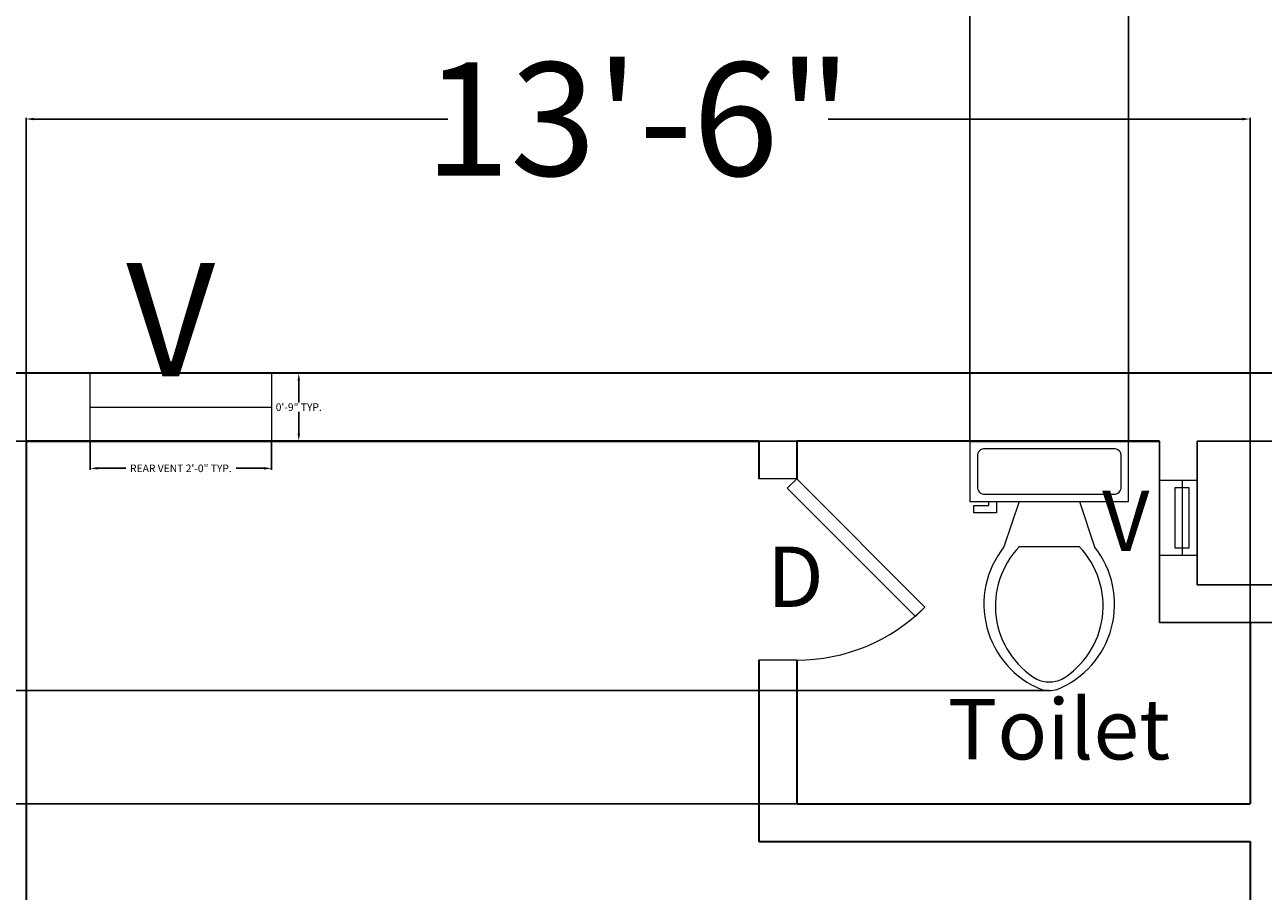
# Model space of a CAD drawing. Units: inches. Extents: x 371 to 1095, y -45 to 1219.
# Tile 16 of 18: x 502 to 666, y 913 to 1028. Entities that reach past the tile are written whole.
import ezdxf

# ---------------------------------------------------------------- set-up
doc = ezdxf.new("R2010")
doc.units = ezdxf.units.IN
doc.header["$MEASUREMENT"] = 0
for name, color, linetype, lineweight in [('A-ANNO-DIMS', 2, 'Continuous', 18), ('A-ANNO-TEXT', 7, 'Continuous', 18), ('A-AREA-IDEN', 7, 'Continuous', 18), ('A-DOOR', 3, 'Continuous', 18), ('A-FLOR-FIXT', 9, 'Continuous', 18), ('A-FLOR-SHFT', 7, 'Continuous', 25), ('A-GLAZ', 4, 'Continuous', 18), ('A-WALL', 40, 'Continuous', 35)]:
    doc.layers.add(name, color=color, linetype=linetype, lineweight=lineweight)
doc.styles.get("Standard").update_dxf_attribs({"font": 'arial.ttf'})
doc.dimstyles.get("Standard").update_dxf_attribs({"dimtxt": 1, "dimasz": 1, "dimexe": 0.18, "dimexo": 0.0625, "dimgap": 0.09, "dimtad": 0, "dimtih": 1, "dimtoh": 1, "dimdec": 0, "dimzin": 0, "dimdsep": 46, "dimlunit": 3, "dimtxsty": 'Standard', "dimcen": 0.09, "dimadec": 0, "dimazin": 0, "dimtfac": 1, "dimtdec": 0, "dimtofl": 0, "dimtmove": 0, "dimatfit": 3, "dimfxl": 1, "dimtolj": 1, "dimtzin": 0, "dimarcsym": 0})

# ---------------------------------------------------------------- blocks, each defined once
blk = doc.blocks.new('*U2')
for p, q in [((9.5, -6), (9.5, -2)), ((-8, -8.5), (-8, -8)), ((-7, -8), (-7, -9.5)), ((-4, -8), (-6, -14)), ((4, -8), (6, -14)), ((-10, -8.5), (-8, -8.5)), ((-10, -9.5), (-10, -8.5)), ((-7, -9.5), (-10, -9.5)), ((4, -14), (-4, -14))]:
    blk.add_line(p, q)
blk.add_lwpolyline([(10.5, -8), (10.5, 0), (-10.5, 0), (-10.5, -8)], close=True)
for points in [[(8.5, -1), (-8.5, -1)], [(-9.5, -2), (-9.5, -6)], [(-8.5, -7), (8.5, -7)]]:
    blk.add_lwpolyline(points)
for centre, radius, start, end in [((-8.62, -1.88), 0.884, 81.8699, 188.1301), ((8.62, -1.88), 0.884, 351.8699, 98.1301), ((-8.62, -6.12), 0.884, 171.8699, 278.1301), ((8.62, -6.12), 0.884, 261.8699, 8.1301), ((3.52, -21.58), 12.17, 141.4691, 247.9714), ((4.2, -21.82), 11.33, 136.3677, 238.9468), ((-3.52, -21.58), 12.17, 292.0284, 38.5307), ((-4.2, -21.82), 11.33, 301.053, 43.6321), ((0, -27.88), 4, 245.7318, 294.2682), ((0, -29), 4, 254.8605, 285.1395)]:
    blk.add_arc(centre, radius, start, end)
blk = doc.blocks.new('*U5')
for p, q in [((0, 0), (0, -5)), ((24, 0), (24, -5))]:
    blk.add_line(p, q)
blk.add_lwpolyline([(0, 0), (16.97, 16.97), (18.21, 15.73), (1.24, -1.24)], close=True)
blk.add_arc((0, 0), 24, 0, 45)
blk = doc.blocks.new('*D8')
at = {"layer": 'A-ANNO-DIMS', "color": 0, "lineweight": -2, "transparency": 16777216}
for p, q in [((501.75, 973.03), (438.47, 973.03)), ((438.65, 972.03), (438.65, 896.65)), ((438.65, 806.03), (438.65, 881.4)), ((501.75, 805.03), (438.47, 805.03))]:
    blk.add_line(p, q, dxfattribs=at)
at = {"layer": 'A-ANNO-DIMS', "color": 0, "transparency": 16777216}
for points in [[(438.48, 972.03), (438.82, 972.03), (438.65, 973.03)], [(438.48, 806.03), (438.82, 806.03), (438.65, 805.03)]]:
    blk.add_solid(points, dxfattribs=at)
at = {"layer": 'Defpoints', "color": 0, "transparency": 16777216}
for p in [(501.81, 973.03), (438.65, 805.03), (501.81, 805.03)]:
    blk.add_point(p, dxfattribs=at)
at = {"layer": 'A-ANNO-DIMS', "color": 0, "transparency": 16777216, "insert": (438.65, 889.03), "char_height": 1, "attachment_point": 5}
blk.add_mtext("\\A1;{\\H15x;14'}", dxfattribs=at)
blk = doc.blocks.new('*D19')
at = {"layer": 'A-ANNO-DIMS', "color": 0, "lineweight": -2, "transparency": 16777216}
for p, q in [((501.75, 982.03), (438.6, 982.03)), ((438.78, 981.03), (438.78, 974.03)), ((438.78, 972.03), (437.78, 972.03)), ((501.75, 973.03), (438.6, 973.03)), ((438.78, 973.03), (438.78, 972.03))]:
    blk.add_line(p, q, dxfattribs=at)
at = {"layer": 'A-ANNO-DIMS', "color": 0, "transparency": 16777216}
for points in [[(438.62, 981.03), (438.95, 981.03), (438.78, 982.03)], [(438.62, 974.03), (438.95, 974.03), (438.78, 973.03)]]:
    blk.add_solid(points, dxfattribs=at)
at = {"layer": 'Defpoints', "color": 0, "transparency": 16777216}
for p in [(501.81, 982.03), (438.78, 973.03), (501.81, 973.03)]:
    blk.add_point(p, dxfattribs=at)
at = {"layer": 'A-ANNO-DIMS', "color": 0, "transparency": 16777216, "insert": (429.07, 972.03), "char_height": 1, "attachment_point": 5}
blk.add_mtext('\\A1;{\\H15x;9"}', dxfattribs=at)
blk = doc.blocks.new('*D26')
at = {"layer": 'A-ANNO-DIMS', "color": 0, "lineweight": -2, "transparency": 16777216}
for p, q in [((501.81, 949.09), (501.81, 1015.85)), ((502.81, 1015.67), (557.66, 1015.67)), ((662.81, 1015.67), (607.96, 1015.67)), ((663.81, 949.09), (663.81, 1015.85))]:
    blk.add_line(p, q, dxfattribs=at)
at = {"layer": 'A-ANNO-DIMS', "color": 0, "transparency": 16777216}
for points in [[(502.81, 1015.84), (502.81, 1015.51), (501.81, 1015.67)], [(662.81, 1015.84), (662.81, 1015.51), (663.81, 1015.67)]]:
    blk.add_solid(points, dxfattribs=at)
at = {"layer": 'Defpoints', "color": 0, "transparency": 16777216}
for p in [(501.81, 1015.67), (501.81, 949.03), (663.81, 949.03)]:
    blk.add_point(p, dxfattribs=at)
at = {"layer": 'A-ANNO-DIMS', "color": 0, "transparency": 16777216, "insert": (582.81, 1015.67), "char_height": 1, "attachment_point": 5}
blk.add_mtext('\\A1;{\\H15x;13\'-6"}', dxfattribs=at)
blk = doc.blocks.new('VENT-24-REAR')
blk.add_line((0, 4.5), (24, 4.5))
blk.add_lwpolyline([(0, 9), (24, 9), (24, 0), (0, 0)], close=True)
blk = doc.blocks.new('VENT-DUCT-SASH')
blk.add_line((0.9, 10), (0.9, 0))
blk.add_lwpolyline([(1.79, 9), (1.79, 1), (0, 1), (0, 9)], close=True)
blk = doc.blocks.new('SHAFT-REAR')
for p, q in [((0, 24), (0, 0)), ((5, 24), (5, 5)), ((28, 24), (5, 24)), ((28, 24), (28, 5)), ((33, 24), (33, 0)), ((5, 5), (28, 5)), ((0, 0), (33, 0))]:
    blk.add_line(p, q)
blk = doc.blocks.new('*D40')
at = {"layer": 'A-ANNO-DIMS', "color": 0, "lineweight": -2, "transparency": 16777216}
for p, q in [((510.31, 972.96), (510.31, 969.25)), ((534.31, 972.96), (534.31, 969.25)), ((511.31, 969.43), (515.01, 969.43)), ((533.31, 969.43), (529.62, 969.43))]:
    blk.add_line(p, q, dxfattribs=at)
at = {"layer": 'A-ANNO-DIMS', "color": 0, "transparency": 16777216}
for points in [[(511.31, 969.59), (511.31, 969.26), (510.31, 969.43)], [(533.31, 969.59), (533.31, 969.26), (534.31, 969.43)]]:
    blk.add_solid(points, dxfattribs=at)
at = {"layer": 'Defpoints', "color": 0, "transparency": 16777216}
for p in [(510.31, 973.03), (534.31, 973.03), (534.31, 969.43)]:
    blk.add_point(p, dxfattribs=at)
at = {"layer": 'A-ANNO-DIMS', "color": 0, "transparency": 16777216, "insert": (522.31, 969.43), "char_height": 1, "attachment_point": 5}
blk.add_mtext('\\A1;REAR VENT 2\'-0" TYP.', dxfattribs=at)
blk = doc.blocks.new('*D41')
at = {"layer": 'A-ANNO-DIMS', "color": 0, "lineweight": -2, "transparency": 16777216}
for p, q in [((534.38, 982.03), (538.09, 982.03)), ((537.91, 981.03), (537.91, 978.13)), ((537.91, 974.03), (537.91, 976.92)), ((534.38, 973.03), (538.09, 973.03))]:
    blk.add_line(p, q, dxfattribs=at)
at = {"layer": 'A-ANNO-DIMS', "color": 0, "transparency": 16777216}
for points in [[(537.75, 981.03), (538.08, 981.03), (537.91, 982.03)], [(537.75, 974.03), (538.08, 974.03), (537.91, 973.03)]]:
    blk.add_solid(points, dxfattribs=at)
at = {"layer": 'Defpoints', "color": 0, "transparency": 16777216}
for p in [(534.31, 982.03), (537.91, 982.03), (534.31, 973.03)]:
    blk.add_point(p, dxfattribs=at)
at = {"layer": 'A-ANNO-DIMS', "color": 0, "transparency": 16777216, "insert": (537.91, 977.53), "char_height": 1, "attachment_point": 5}
blk.add_mtext('\\A1;0\'-9" TYP.', dxfattribs=at)
blk = doc.blocks.new('*D50')
at = {"layer": 'A-ANNO-DIMS', "color": 0, "lineweight": -2, "transparency": 16777216}
for p, q in [((492.81, 982.09), (492.81, 1093.41)), ((1032.81, 982.09), (1032.81, 1093.41)), ((493.81, 1093.23), (760.98, 1093.23)), ((1031.81, 1093.23), (764.64, 1093.23))]:
    blk.add_line(p, q, dxfattribs=at)
at = {"layer": 'A-ANNO-DIMS', "color": 0, "transparency": 16777216}
for points in [[(493.81, 1093.39), (493.81, 1093.06), (492.81, 1093.23)], [(1031.81, 1093.39), (1031.81, 1093.06), (1032.81, 1093.23)]]:
    blk.add_solid(points, dxfattribs=at)
at = {"layer": 'Defpoints', "color": 0, "transparency": 16777216}
for p in [(1032.81, 1093.23), (492.81, 982.03), (1032.81, 982.03)]:
    blk.add_point(p, dxfattribs=at)
at = {"layer": 'A-ANNO-DIMS', "color": 0, "transparency": 16777216, "insert": (762.81, 1093.23), "char_height": 1, "attachment_point": 5}
blk.add_mtext('\\A1;45\'-0"', dxfattribs=at)
blk = doc.blocks.new('*D55')
at = {"layer": 'A-ANNO-DIMS', "color": 0, "lineweight": -2, "transparency": 16777216}
for p, q in [((603.75, 973.03), (432.43, 973.03)), ((432.61, 972.03), (432.61, 949.63)), ((432.61, 926.03), (432.61, 948.42)), ((603.75, 925.03), (432.43, 925.03))]:
    blk.add_line(p, q, dxfattribs=at)
at = {"layer": 'A-ANNO-DIMS', "color": 0, "transparency": 16777216}
for points in [[(432.44, 972.03), (432.77, 972.03), (432.61, 973.03)], [(432.44, 926.03), (432.77, 926.03), (432.61, 925.03)]]:
    blk.add_solid(points, dxfattribs=at)
at = {"layer": 'Defpoints', "color": 0, "transparency": 16777216}
for p in [(432.61, 973.03), (603.81, 973.03), (603.81, 925.03)]:
    blk.add_point(p, dxfattribs=at)
at = {"layer": 'A-ANNO-DIMS', "color": 0, "transparency": 16777216, "insert": (432.61, 949.03), "char_height": 1, "attachment_point": 5}
blk.add_mtext('\\A1;4\'-0"', dxfattribs=at)
blk = doc.blocks.new('*D58')
at = {"layer": 'A-ANNO-DIMS', "color": 0, "lineweight": -2, "transparency": 16777216}
for p, q in [((626.74, 973.09), (626.74, 1093.41)), ((647.74, 973.09), (647.74, 1093.41)), ((627.74, 1093.23), (635.86, 1093.23)), ((646.74, 1093.23), (638.61, 1093.23))]:
    blk.add_line(p, q, dxfattribs=at)
at = {"layer": 'A-ANNO-DIMS', "color": 0, "transparency": 16777216}
for points in [[(627.74, 1093.39), (627.74, 1093.06), (626.74, 1093.23)], [(646.74, 1093.39), (646.74, 1093.06), (647.74, 1093.23)]]:
    blk.add_solid(points, dxfattribs=at)
at = {"layer": 'Defpoints', "color": 0, "transparency": 16777216}
for p in [(647.74, 1093.23), (626.74, 973.03), (647.74, 973.03)]:
    blk.add_point(p, dxfattribs=at)
at = {"layer": 'A-ANNO-DIMS', "color": 0, "transparency": 16777216, "insert": (637.24, 1093.23), "char_height": 1, "attachment_point": 5}
blk.add_mtext('\\A1;1\'-9"', dxfattribs=at)
blk = doc.blocks.new('*D59')
at = {"layer": 'A-ANNO-DIMS', "color": 0, "lineweight": -2, "transparency": 16777216}
for p, q in [((626.67, 973.03), (432.43, 973.03)), ((432.61, 972.03), (432.61, 957.13)), ((432.61, 941.03), (432.61, 955.92)), ((637.17, 940.03), (432.43, 940.03))]:
    blk.add_line(p, q, dxfattribs=at)
at = {"layer": 'A-ANNO-DIMS', "color": 0, "transparency": 16777216}
for points in [[(432.44, 972.03), (432.77, 972.03), (432.61, 973.03)], [(432.44, 941.03), (432.77, 941.03), (432.61, 940.03)]]:
    blk.add_solid(points, dxfattribs=at)
at = {"layer": 'Defpoints', "color": 0, "transparency": 16777216}
for p in [(432.61, 973.03), (626.74, 973.03), (637.24, 940.03)]:
    blk.add_point(p, dxfattribs=at)
at = {"layer": 'A-ANNO-DIMS', "color": 0, "transparency": 16777216, "insert": (432.61, 956.53), "char_height": 1, "attachment_point": 5}
blk.add_mtext('\\A1;2\'-9"', dxfattribs=at)

msp = doc.modelspace()

# ---------------------------------------------------------------- linework, layer by layer
at = {"layer": 'A-GLAZ'}
msp.add_lwpolyline([(656.81, 967.87), (656.81, 957.87), (651.81, 957.87), (651.81, 967.87)], close=True, dxfattribs=at)
at = {"layer": 'A-WALL'}
for p, q in [((1032.81, 982.03), (492.81, 982.03)), ((501.81, 973.02), (501.81, 805.03)), ((501.81, 973.02), (598.81, 973.02)), ((598.81, 973.02), (501.81, 973.02)), ((598.81, 973.02), (598.81, 968.03)), ((651.81, 973.02), (603.81, 973.02)), ((603.81, 973.02), (603.81, 968.03)), ((626.74, 973.02), (651.81, 973.02)), ((663.81, 949.02), (663.81, 925.03)), ((598.81, 944.03), (598.81, 920.03)), ((603.81, 944.03), (603.81, 925.03)), ((603.81, 925.03), (663.81, 925.03)), ((598.81, 920.03), (663.81, 920.03)), ((663.81, 920.03), (663.81, 805.03))]:
    msp.add_line(p, q, dxfattribs=at)

# ---------------------------------------------------------------- block references
at = {"layer": 'A-DOOR', "rotation": 270}
msp.add_blockref('*U5', (603.81, 968.03), dxfattribs=at)
at = {"layer": 'A-FLOR-FIXT'}
msp.add_blockref('*U2', (637.24, 973.02), dxfattribs=at)
at = {"layer": 'A-FLOR-SHFT'}
msp.add_blockref('SHAFT-REAR', (651.81, 949.02), dxfattribs=at)
at = {"layer": 'A-GLAZ'}
for name, p in [('VENT-24-REAR', (510.31, 973.02)), ('VENT-DUCT-SASH', (653.91, 957.87))]:
    msp.add_blockref(name, p, dxfattribs=at)

# ---------------------------------------------------------------- texts
at = {"layer": 'A-ANNO-TEXT', "attachment_point": 1}
for s, insert, char_height in [('V', (515.07, 996.61), 15), ('V', (644.23, 966.48), 8), ('D', (599.89, 959.07), 8)]:
    msp.add_mtext_dynamic_manual_height_columns(s, width=17.4938, gutter_width=1, heights=[0], dxfattribs=dict(at, insert=insert, char_height=char_height))
at = {"layer": 'A-AREA-IDEN', "insert": (623.83, 938.89), "char_height": 8, "attachment_point": 1}
msp.add_mtext_dynamic_manual_height_columns('Toilet', width=31.9108, gutter_width=1, heights=[0], dxfattribs=at)

# ---------------------------------------------------------------- dimensions: what is measured, and where the dimension line sits
at = {"layer": 'A-ANNO-DIMS'}
for base, p1, p2, picture, middle in [((1032.81, 1093.23), (492.81, 982.03), (1032.81, 982.03), '*D50', (762.81, 1093.23)), ((647.74, 1093.23), (626.74, 973.02), (647.74, 973.02), '*D58', (637.24, 1093.23))]:
    dim = msp.add_linear_dim(base=base, p1=p1, p2=p2, dimstyle='Standard', override={"dimdec": 1, "dimlfac": 1, "dimrnd": 0, "dimzin": 1, "dimdsep": 46, "dimlunit": 4, "dimfrac": 2}, dxfattribs=at)
    dim.commit()
    dim.dimension.update_dxf_attribs({"geometry": picture, "text_midpoint": middle})
for base, p1, p2, text, override, picture, middle in [((501.81, 1015.67), (663.81, 949.02), (501.81, 949.02), '{\\H15x;<>}', {"dimclrd": 0, "dimclre": 0, "dimclrt": 0}, '*D26', (582.81, 1015.67)), ((534.31, 969.43), (510.31, 973.02), (534.31, 973.02), 'REAR VENT <> TYP.', {"dimdec": 1, "dimlfac": 1, "dimrnd": 0, "dimzin": 1, "dimdsep": 46, "dimlunit": 4, "dimfrac": 2}, '*D40', (522.31, 969.43))]:
    dim = msp.add_linear_dim(base=base, p1=p1, p2=p2, text=text, dimstyle='Standard', override=override, dxfattribs=at)
    dim.commit()
    dim.dimension.update_dxf_attribs({"geometry": picture, "text_midpoint": middle})
for base, p1, p2, text, override, picture, middle in [((438.78, 973.02), (501.81, 982.03), (501.81, 973.02), '{\\H15x;<>}', {"dimclrd": 0, "dimclre": 0, "dimclrt": 0}, '*D19', (429.07, 972.03)), ((537.91, 982.03), (534.31, 973.02), (534.31, 982.03), '<> TYP.', {"dimdec": 1, "dimlfac": 1, "dimrnd": 0, "dimzin": 1, "dimdsep": 46, "dimlunit": 4, "dimfrac": 2}, '*D41', (537.91, 977.53)), ((438.65, 805.03), (501.81, 973.02), (501.81, 805.03), '{\\H15x;<>}', {"dimclrd": 0, "dimclre": 0, "dimclrt": 0}, '*D8', (438.65, 889.03))]:
    dim = msp.add_linear_dim(base=base, p1=p1, p2=p2, angle=90, text=text, dimstyle='Standard', override=override, dxfattribs=at)
    dim.commit()
    dim.dimension.update_dxf_attribs({"geometry": picture, "text_midpoint": middle})
for p1, p2, picture, middle in [((603.81, 925.03), (603.81, 973.02), '*D55', (432.61, 949.03)), ((637.24, 940.03), (626.74, 973.02), '*D59', (432.61, 956.53))]:
    dim = msp.add_linear_dim(base=(432.61, 973.02), p1=p1, p2=p2, angle=90, dimstyle='Standard', override={"dimdec": 1, "dimlfac": 1, "dimrnd": 0, "dimzin": 1, "dimdsep": 46, "dimlunit": 4, "dimfrac": 2}, dxfattribs=at)
    dim.commit()
    dim.dimension.update_dxf_attribs({"geometry": picture, "text_midpoint": middle})

doc.saveas('drawing.dxf')
